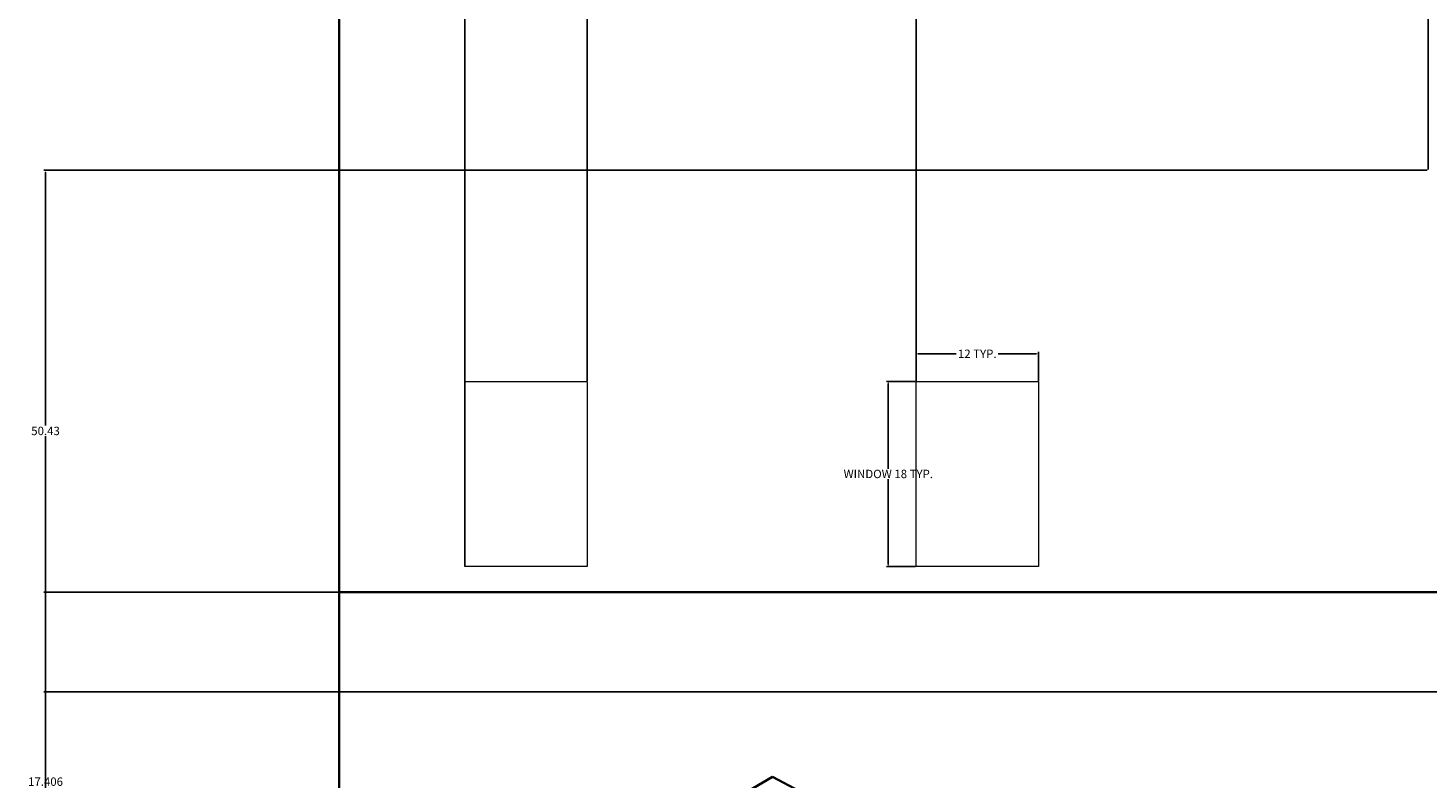
# Model space of a CAD drawing. Units: inches. Extents: x 69 to 650, y -16 to 573.
# Tile 15 of 26: x 69 to 205, y 394 to 466. Entities that reach past the tile are written whole.
import ezdxf

# ---------------------------------------------------------------- set-up
doc = ezdxf.new("R2010")
doc.units = ezdxf.units.IN
doc.header["$MEASUREMENT"] = 0
for name, color, linetype, lineweight in [('A-ANNO-DIMS', 2, 'Continuous', 18), ('A-GLAZ', 4, 'Continuous', 18), ('A-ROOF', 7, 'Continuous', 35), ('A-WALL', 7, 'Continuous', 35)]:
    doc.layers.add(name, color=color, linetype=linetype, lineweight=lineweight)
doc.styles.get("Standard").update_dxf_attribs({"font": 'arial.ttf'})
doc.dimstyles.get("Standard").update_dxf_attribs({"dimtxt": 0.8125, "dimasz": 0.18, "dimexe": 0.18, "dimexo": 0.0625, "dimgap": 0.09, "dimtad": 0, "dimtih": 1, "dimtoh": 1, "dimdec": 4, "dimzin": 0, "dimdsep": 46, "dimlunit": 4, "dimtxsty": 'Standard', "dimcen": 0.09, "dimadec": 0, "dimazin": 0, "dimtfac": 1, "dimtdec": 4, "dimtofl": 0, "dimtmove": 0, "dimatfit": 3, "dimfxl": 1, "dimtolj": 1, "dimtzin": 0, "dimarcsym": 0})

# ---------------------------------------------------------------- blocks, each defined once
blk = doc.blocks.new('CAP-SIDE-PEDIMENT')
for p, q in [((39.09, 30.19), (2.58, 11)), ((71.85, 11), (39.09, 30.19)), ((78.18, 11), (0, 11)), ((0, 11), (0, 9.99)), ((0, 9.99), (2.58, 9.99)), ((71.82, 9.99), (2.58, 9.99)), ((2.58, 9.99), (2.58, 0)), ((71.82, 0), (71.82, 9.99)), ((71.82, 9.99), (78.18, 9.99))]:
    blk.add_line(p, q)
blk = doc.blocks.new('WIN-UPPER-SMALL')
blk.add_lwpolyline([(0, 17.88), (11.84, 17.88), (11.84, 0), (0, 0)], close=True)
blk = doc.blocks.new('*D7')
at = {"layer": 'A-ANNO-DIMS', "color": 0, "lineweight": -2, "transparency": 16777216}
for p, q in [((155.29, 432.3), (152.49, 432.3)), ((152.67, 432.12), (152.67, 423.87)), ((152.67, 414.59), (152.67, 422.84)), ((155.29, 414.41), (152.49, 414.41))]:
    blk.add_line(p, q, dxfattribs=at)
at = {"layer": 'A-ANNO-DIMS', "color": 0, "transparency": 16777216}
for points in [[(152.64, 432.12), (152.7, 432.12), (152.67, 432.3)], [(152.64, 414.59), (152.7, 414.59), (152.67, 414.41)]]:
    blk.add_solid(points, dxfattribs=at)
at = {"layer": 'Defpoints', "color": 0, "transparency": 16777216}
for p in [(152.67, 432.3), (155.35, 432.3), (155.35, 414.41)]:
    blk.add_point(p, dxfattribs=at)
at = {"layer": 'A-ANNO-DIMS', "color": 0, "transparency": 16777216, "insert": (152.67, 423.36), "char_height": 0.8125, "attachment_point": 5}
blk.add_mtext('\\A1;WINDOW 18 TYP.', dxfattribs=at)
blk = doc.blocks.new('*D8')
at = {"layer": 'A-ANNO-DIMS', "color": 0, "lineweight": -2, "transparency": 16777216}
for p, q in [((155.35, 432.36), (155.35, 435.16)), ((155.53, 434.98), (159.24, 434.98)), ((167.01, 434.98), (163.3, 434.98)), ((167.19, 432.36), (167.19, 435.16))]:
    blk.add_line(p, q, dxfattribs=at)
at = {"layer": 'A-ANNO-DIMS', "color": 0, "transparency": 16777216}
for points in [[(155.53, 435.01), (155.53, 434.95), (155.35, 434.98)], [(167.01, 435.01), (167.01, 434.95), (167.19, 434.98)]]:
    blk.add_solid(points, dxfattribs=at)
at = {"layer": 'Defpoints', "color": 0, "transparency": 16777216}
for p in [(167.19, 434.98), (155.35, 432.3), (167.19, 432.3)]:
    blk.add_point(p, dxfattribs=at)
at = {"layer": 'A-ANNO-DIMS', "color": 0, "transparency": 16777216, "insert": (161.27, 434.98), "char_height": 0.8125, "attachment_point": 5}
blk.add_mtext('\\A1;12 TYP.', dxfattribs=at)
blk = doc.blocks.new('*D19')
at = {"layer": 'A-ANNO-DIMS', "color": 0, "lineweight": -2, "transparency": 16777216}
for p, q in [((99.56, 471.72), (99.56, 572.74)), ((99.74, 572.56), (358.57, 572.56)), ((619.38, 572.56), (360.54, 572.56)), ((619.56, 87.99), (619.56, 572.74))]:
    blk.add_line(p, q, dxfattribs=at)
at = {"layer": 'A-ANNO-DIMS', "color": 0, "transparency": 16777216}
for points in [[(99.74, 572.59), (99.74, 572.53), (99.56, 572.56)], [(619.38, 572.59), (619.38, 572.53), (619.56, 572.56)]]:
    blk.add_solid(points, dxfattribs=at)
at = {"layer": 'Defpoints', "color": 0, "transparency": 16777216}
for p in [(619.56, 572.56), (99.56, 471.66), (619.56, 87.93)]:
    blk.add_point(p, dxfattribs=at)
at = {"layer": 'A-ANNO-DIMS', "color": 0, "transparency": 16777216, "insert": (359.56, 572.56), "char_height": 0.812, "attachment_point": 5}
blk.add_mtext('\\A1;520', dxfattribs=at)
blk = doc.blocks.new('*D47')
at = {"layer": 'A-ANNO-DIMS', "color": 0, "lineweight": -2, "transparency": 16777216}
for p, q in [((99.49, 411.93), (70.98, 411.93)), ((71.16, 411.75), (71.16, 388.41)), ((71.16, 364.05), (71.16, 387.4)), ((99.49, 363.87), (70.98, 363.87))]:
    blk.add_line(p, q, dxfattribs=at)
at = {"layer": 'A-ANNO-DIMS', "color": 0, "transparency": 16777216}
for points in [[(71.13, 411.75), (71.19, 411.75), (71.16, 411.93)], [(71.13, 364.05), (71.19, 364.05), (71.16, 363.87)]]:
    blk.add_solid(points, dxfattribs=at)
at = {"layer": 'Defpoints', "color": 0, "transparency": 16777216}
for p in [(71.16, 411.93), (99.56, 411.93), (99.56, 363.87)]:
    blk.add_point(p, dxfattribs=at)
at = {"layer": 'A-ANNO-DIMS', "color": 0, "transparency": 16777216, "insert": (71.16, 387.9), "char_height": 0.812, "attachment_point": 5}
blk.add_mtext('\\A1;48.06', dxfattribs=at)
blk = doc.blocks.new('*D53')
at = {"layer": 'A-ANNO-DIMS', "color": 0, "lineweight": -2, "transparency": 16777216}
for p, q in [((99.56, 411.99), (99.56, 572.74)), ((99.74, 572.56), (103.9, 572.56)), ((111.53, 572.56), (107.37, 572.56)), ((111.71, 414.48), (111.71, 572.74))]:
    blk.add_line(p, q, dxfattribs=at)
at = {"layer": 'A-ANNO-DIMS', "color": 0, "transparency": 16777216}
for points in [[(99.74, 572.59), (99.74, 572.53), (99.56, 572.56)], [(111.53, 572.59), (111.53, 572.53), (111.71, 572.56)]]:
    blk.add_solid(points, dxfattribs=at)
at = {"layer": 'Defpoints', "color": 0, "transparency": 16777216}
for p in [(111.71, 572.56), (111.71, 414.41), (99.56, 411.93)]:
    blk.add_point(p, dxfattribs=at)
at = {"layer": 'A-ANNO-DIMS', "color": 0, "transparency": 16777216, "insert": (105.63, 572.56), "char_height": 0.812, "attachment_point": 5}
blk.add_mtext('\\A1;12.156', dxfattribs=at)
blk = doc.blocks.new('*D54')
at = {"layer": 'A-ANNO-DIMS', "color": 0, "lineweight": -2, "transparency": 16777216}
for p, q in [((123.55, 432.36), (123.55, 572.74)), ((123.73, 572.56), (138.31, 572.56)), ((155.17, 572.56), (140.6, 572.56)), ((155.35, 432.36), (155.35, 572.74))]:
    blk.add_line(p, q, dxfattribs=at)
at = {"layer": 'A-ANNO-DIMS', "color": 0, "transparency": 16777216}
for points in [[(123.73, 572.59), (123.73, 572.53), (123.55, 572.56)], [(155.17, 572.59), (155.17, 572.53), (155.35, 572.56)]]:
    blk.add_solid(points, dxfattribs=at)
at = {"layer": 'Defpoints', "color": 0, "transparency": 16777216}
for p in [(155.35, 572.56), (123.55, 432.3), (155.35, 432.3)]:
    blk.add_point(p, dxfattribs=at)
at = {"layer": 'A-ANNO-DIMS', "color": 0, "transparency": 16777216, "insert": (139.45, 572.56), "char_height": 0.812, "attachment_point": 5}
blk.add_mtext('\\A1;31.8', dxfattribs=at)
blk = doc.blocks.new('*D59')
at = {"layer": 'A-ANNO-DIMS', "color": 0, "lineweight": -2, "transparency": 16777216}
for p, q in [((214.82, 402.3), (70.98, 402.3)), ((71.16, 402.12), (71.16, 394.11)), ((71.16, 385.08), (71.16, 393.1)), ((307.73, 384.9), (70.98, 384.9))]:
    blk.add_line(p, q, dxfattribs=at)
at = {"layer": 'A-ANNO-DIMS', "color": 0, "transparency": 16777216}
for points in [[(71.13, 402.12), (71.19, 402.12), (71.16, 402.3)], [(71.13, 385.08), (71.19, 385.08), (71.16, 384.9)]]:
    blk.add_solid(points, dxfattribs=at)
at = {"layer": 'Defpoints', "color": 0, "transparency": 16777216}
for p in [(71.16, 402.3), (214.89, 402.3), (307.8, 384.9)]:
    blk.add_point(p, dxfattribs=at)
at = {"layer": 'A-ANNO-DIMS', "color": 0, "transparency": 16777216, "insert": (71.16, 393.6), "char_height": 0.812, "attachment_point": 5}
blk.add_mtext('\\A1;17.406', dxfattribs=at)
blk = doc.blocks.new('*D60')
at = {"layer": 'A-ANNO-DIMS', "color": 0, "lineweight": -2, "transparency": 16777216}
for p, q in [((204.8, 452.74), (70.98, 452.74)), ((71.16, 452.56), (71.16, 428.03)), ((71.16, 402.48), (71.16, 427.02)), ((214.82, 402.3), (70.98, 402.3))]:
    blk.add_line(p, q, dxfattribs=at)
at = {"layer": 'A-ANNO-DIMS', "color": 0, "transparency": 16777216}
for points in [[(71.13, 452.56), (71.19, 452.56), (71.16, 452.74)], [(71.13, 402.48), (71.19, 402.48), (71.16, 402.3)]]:
    blk.add_solid(points, dxfattribs=at)
at = {"layer": 'Defpoints', "color": 0, "transparency": 16777216}
for p in [(71.16, 452.74), (204.87, 452.74), (214.89, 402.3)]:
    blk.add_point(p, dxfattribs=at)
at = {"layer": 'A-ANNO-DIMS', "color": 0, "transparency": 16777216, "insert": (71.16, 427.52), "char_height": 0.812, "attachment_point": 5}
blk.add_mtext('\\A1;50.43', dxfattribs=at)
blk = doc.blocks.new('*D61')
at = {"layer": 'A-ANNO-DIMS', "color": 0, "lineweight": -2, "transparency": 16777216}
for p, q in [((99.56, 471.72), (99.56, 572.74)), ((99.74, 572.56), (150.79, 572.56)), ((204.69, 572.56), (153.63, 572.56)), ((204.87, 452.8), (204.87, 572.74))]:
    blk.add_line(p, q, dxfattribs=at)
at = {"layer": 'A-ANNO-DIMS', "color": 0, "transparency": 16777216}
for points in [[(99.74, 572.59), (99.74, 572.53), (99.56, 572.56)], [(204.69, 572.59), (204.69, 572.53), (204.87, 572.56)]]:
    blk.add_solid(points, dxfattribs=at)
at = {"layer": 'Defpoints', "color": 0, "transparency": 16777216}
for p in [(204.87, 572.56), (99.56, 471.66), (204.87, 452.74)]:
    blk.add_point(p, dxfattribs=at)
at = {"layer": 'A-ANNO-DIMS', "color": 0, "transparency": 16777216, "insert": (152.21, 572.56), "char_height": 0.812, "attachment_point": 5}
blk.add_mtext('\\A1;105.3', dxfattribs=at)
blk = doc.blocks.new('*D62')
at = {"layer": 'A-ANNO-DIMS', "color": 0, "lineweight": -2, "transparency": 16777216}
for p, q in [((204.87, 452.8), (204.87, 572.74)), ((205.05, 572.56), (356.52, 572.56)), ((510.91, 572.56), (359.44, 572.56)), ((511.09, 451.98), (511.09, 572.74))]:
    blk.add_line(p, q, dxfattribs=at)
at = {"layer": 'A-ANNO-DIMS', "color": 0, "transparency": 16777216}
for points in [[(205.05, 572.59), (205.05, 572.53), (204.87, 572.56)], [(510.91, 572.59), (510.91, 572.53), (511.09, 572.56)]]:
    blk.add_solid(points, dxfattribs=at)
at = {"layer": 'Defpoints', "color": 0, "transparency": 16777216}
for p in [(511.09, 572.56), (204.87, 452.74), (511.09, 451.92)]:
    blk.add_point(p, dxfattribs=at)
at = {"layer": 'A-ANNO-DIMS', "color": 0, "transparency": 16777216, "insert": (357.98, 572.56), "char_height": 0.812, "attachment_point": 5}
blk.add_mtext('\\A1;306.2', dxfattribs=at)

msp = doc.modelspace()

# ---------------------------------------------------------------- linework, layer by layer
at = {"layer": 'A-WALL'}
for p, q in [((99.556, 411.93), (99.556, 471.6595)), ((99.556, 243.93), (99.556, 411.93)), ((99.556, 411.93), (619.555, 411.93))]:
    msp.add_line(p, q, dxfattribs=at)

# ---------------------------------------------------------------- block references
at = {"layer": 'A-GLAZ'}
for p in [(111.712, 414.415), (155.3536, 414.415)]:
    msp.add_blockref('WIN-UPPER-SMALL', p, dxfattribs=at)
at = {"layer": 'A-ROOF', "extrusion": (0, 0, -1), "zscale": -1}
msp.add_blockref('CAP-SIDE-PEDIMENT', (-180.548, 363.874), dxfattribs=at)

# ---------------------------------------------------------------- dimensions: what is measured, and where the dimension line sits
at = {"layer": 'A-ANNO-DIMS'}
for base, p1, p2, override, picture, middle in [((619.555, 572.5573), (99.556, 471.6595), (619.555, 87.93), {"dimdec": 0, "dimlfac": 1, "dimrnd": 0, "dimzin": 0, "dimdsep": 46, "dimlunit": 2}, '*D19', (359.5555, 572.5573)), ((111.7119, 572.5573), (99.556, 411.93), (111.7119, 414.4146), {"dimdec": 3, "dimlfac": 1, "dimrnd": 0, "dimzin": 0, "dimdsep": 46, "dimlunit": 2}, '*D53', (105.634, 572.5573)), ((204.8658, 572.5573), (99.556, 471.6595), (204.8658, 452.7384), {"dimdec": 1, "dimlfac": 1, "dimrnd": 0, "dimzin": 0, "dimdsep": 46, "dimlunit": 2}, '*D61', (152.2109, 572.5573)), ((155.3536, 572.5573), (123.5533, 432.2961), (155.3536, 432.2961), {"dimdec": 1, "dimlfac": 1, "dimrnd": 0, "dimzin": 0, "dimdsep": 46, "dimlunit": 2}, '*D54', (139.4534, 572.5573)), ((511.0913, 572.5573), (204.8658, 452.7384), (511.0913, 451.9213), {"dimdec": 1, "dimlfac": 1, "dimrnd": 0, "dimzin": 0, "dimdsep": 46, "dimlunit": 2}, '*D62', (357.9786, 572.5573))]:
    dim = msp.add_linear_dim(base=base, p1=p1, p2=p2, dimstyle='Standard', override=override, dxfattribs=at)
    dim.commit()
    dim.dimension.update_dxf_attribs({"geometry": picture, "text_midpoint": middle})
for base, p1, p2, override, picture, middle in [((71.156, 452.7384), (214.8863, 402.3042), (204.8658, 452.7384), {"dimdec": 2, "dimlfac": 1, "dimrnd": 0, "dimzin": 0, "dimdsep": 46, "dimlunit": 2}, '*D60', (71.156, 427.5213)), ((71.156, 411.93), (99.556, 363.8739), (99.556, 411.93), {"dimdec": 2, "dimlfac": 1, "dimrnd": 0, "dimzin": 0, "dimdsep": 46, "dimlunit": 2}, '*D47', (71.156, 387.902)), ((71.156, 402.3042), (307.7955, 384.8986), (214.8863, 402.3042), {"dimdec": 3, "dimlfac": 1, "dimrnd": 0, "dimzin": 0, "dimdsep": 46, "dimlunit": 2}, '*D59', (71.156, 393.6014))]:
    dim = msp.add_linear_dim(base=base, p1=p1, p2=p2, angle=90, dimstyle='Standard', override=override, dxfattribs=at)
    dim.commit()
    dim.dimension.update_dxf_attribs({"geometry": picture, "text_midpoint": middle})
dim = msp.add_linear_dim(base=(167.1949, 434.9784), p1=(155.3536, 432.2961), p2=(167.1949, 432.2961), text='<> TYP.', dimstyle='Standard', override={"dimdec": 0, "dimlfac": 1, "dimrnd": 0, "dimzin": 0, "dimdsep": 46, "dimlunit": 2}, dxfattribs=at)
dim.commit()
dim.dimension.update_dxf_attribs({"geometry": '*D8', "text_midpoint": (161.2742, 434.9784)})
dim = msp.add_linear_dim(base=(152.6713, 432.2961), p1=(155.3536, 414.4146), p2=(155.3536, 432.2961), angle=90, text='WINDOW <> TYP.', dimstyle='Standard', override={"dimdec": 0, "dimlfac": 1, "dimrnd": 0, "dimzin": 0, "dimdsep": 46, "dimlunit": 2}, dxfattribs=at)
dim.commit()
dim.dimension.update_dxf_attribs({"geometry": '*D7', "text_midpoint": (152.6713, 423.3553)})

doc.saveas('drawing.dxf')
